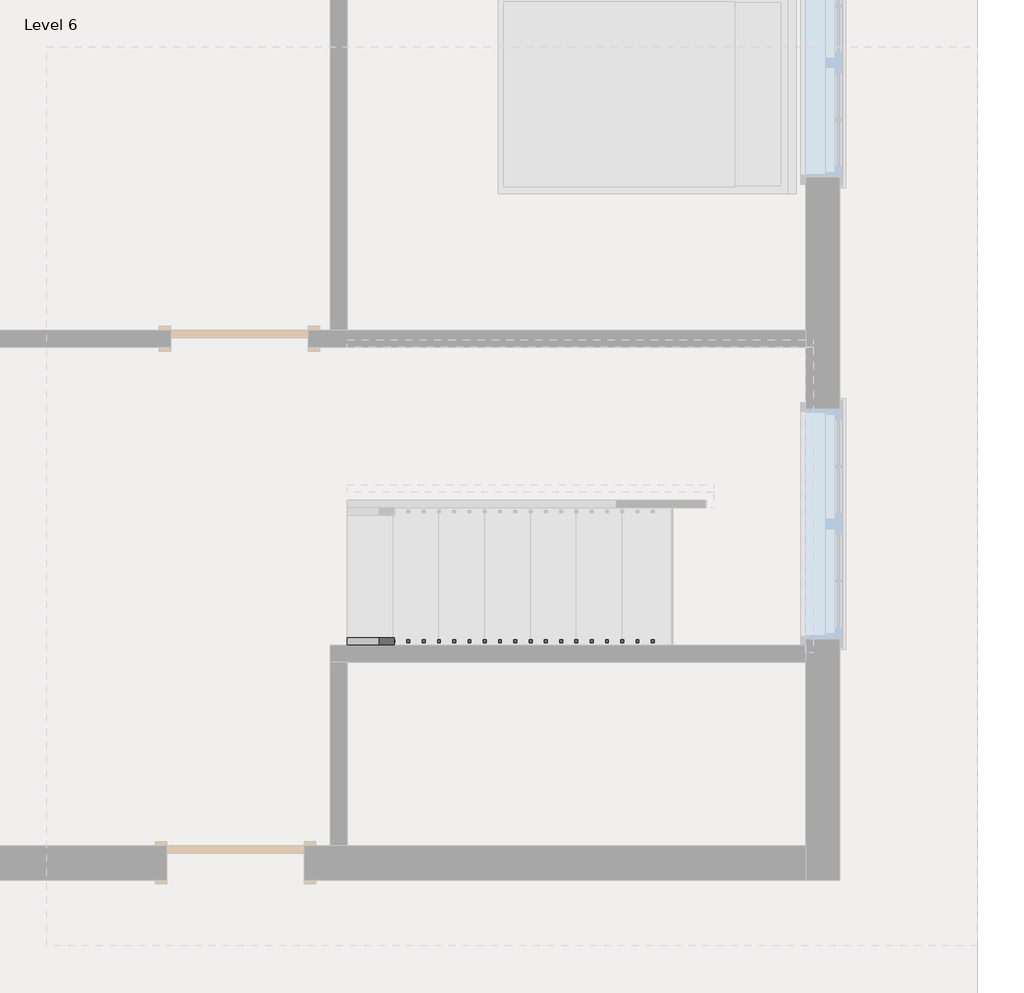
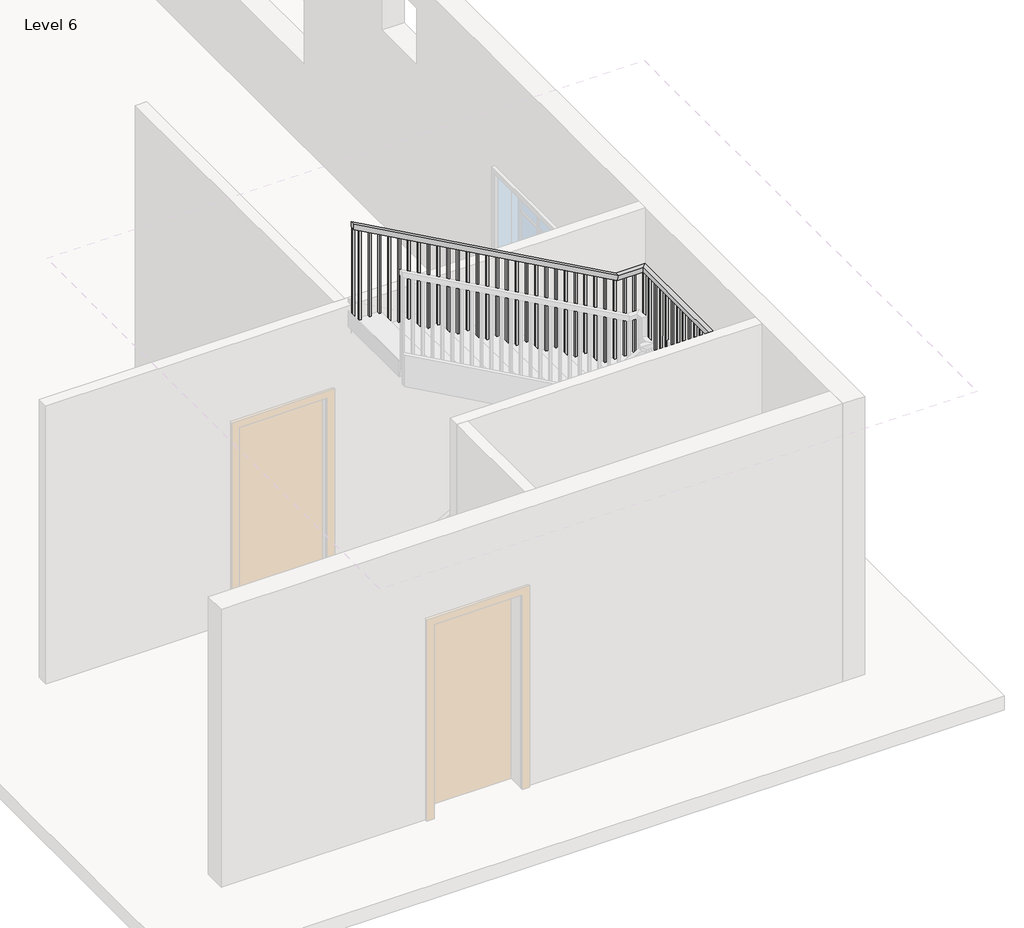
# One storey, part 2 of 3: 1 railing.
"""IFC4 building model written with IfcOpenShell, lengths in millimetres."""

from ifc_helpers import new_model, si_unit, frame, origin, place, context, project, spatial, polyline, outline, extrude, faceted_brep, element, save

model = new_model("IFC4")

# Units and contexts
model_context = context("Model", 3, world=origin())
ifc_project = project(units=[si_unit("LENGTHUNIT", "METRE", prefix="MILLI")], contexts=[model_context])

# Site, building, storey
site = spatial("IfcSite", under=ifc_project)
building = spatial("IfcBuilding", under=site)
storey = spatial("IfcBuildingStorey", under=building, Name="Level 6", Elevation=15849.6)

# Railing
placement = place(None, origin())
element("IfcRailing", 1, ObjectType="Handrail - Rectangular", at=placement, inside=storey, context=model_context, shape_type="SolidModel", body=[
    faceted_brep([(-1197.97188, -4765.70869, 16933.3333333), (-1197.97188, -4765.70869, 16875.220221), (-1197.97188, -4816.50869, 16875.220221), (-1197.97188, -4816.50869, 16933.3333333), (1240.42812, -4765.70869, 18288.0), (1253.5917222, -4765.70869, 18237.2), (1253.5917222, -4816.50869, 18237.2), (1240.42812, -4816.50869, 18288.0), (1799.22812, -4765.70869, 18288.0), (1799.22812, -4765.70869, 18237.2), (1850.02812, -4816.50869, 18237.2), (1850.02812, -4816.50869, 18288.0), (1799.22812, -2886.10869, 18288.0), (1799.22812, -2886.10869, 18237.2), (1850.02812, -2835.30869, 18237.2), (1850.02812, -2835.30869, 18288.0), (1545.22812, -2886.10869, 18288.0), (1532.0645177, -2886.10869, 18237.2), (1532.0645177, -2835.30869, 18237.2), (1545.22812, -2835.30869, 18288.0), (-1197.97188, -2886.10869, 19812.0), (-1197.97188, -2835.30869, 19812.0), (-1197.97188, -2835.30869, 19753.8868876), (-1197.97188, -2886.10869, 19753.8868876)], [[[0, 1, 2, 3]], [[1, 0, 4, 5]], [[2, 1, 5, 6]], [[3, 2, 6, 7]], [[0, 3, 7, 4]], [[5, 4, 8, 9]], [[6, 5, 9, 10]], [[7, 6, 10, 11]], [[4, 7, 11, 8]], [[9, 8, 12, 13]], [[10, 9, 13, 14]], [[11, 10, 14, 15]], [[8, 11, 15, 12]], [[13, 12, 16, 17]], [[14, 13, 17, 18]], [[15, 14, 18, 19]], [[12, 15, 19, 16]], [[20, 21, 22, 23]], [[17, 16, 20, 23]], [[18, 17, 23, 22]], [[19, 18, 22, 21]], [[16, 19, 21, 20]]]),
    extrude(outline(polyline([(19706.2618876, -1112.24688), (19716.845221, -1131.29688), (18728.2666667, -1131.29688), (18728.2666667, -1112.24688), (19706.2618876, -1112.24688)])), frame((0.0, -2870.23369, 0.0), z_axis=(0.0, 1.0, 0.0), x_axis=(0.0, 0.0, 1.0)), (0.0, 0.0, 1.0), 19.05),
    extrude(outline(polyline([(19649.8174432, -1010.64688), (19660.4007765, -1029.69688), (18728.2666667, -1029.69688), (18728.2666667, -1010.64688), (19649.8174432, -1010.64688)])), frame((0.0, -2870.23369, 0.0), z_axis=(0.0, 1.0, 0.0), x_axis=(0.0, 0.0, 1.0)), (0.0, 0.0, 1.0), 19.05),
    extrude(outline(polyline([(19593.3729988, -909.04688), (19603.9563321, -928.09688), (18728.2666667, -928.09688), (18728.2666667, -909.04688), (19593.3729988, -909.04688)])), frame((0.0, -2870.23369, 0.0), z_axis=(0.0, 1.0, 0.0), x_axis=(0.0, 0.0, 1.0)), (0.0, 0.0, 1.0), 19.05),
    extrude(outline(polyline([(19536.9285543, -807.44688), (19547.5118876, -826.49688), (18558.9333333, -826.49688), (18558.9333333, -807.44688), (19536.9285543, -807.44688)])), frame((0.0, -2870.23369, 0.0), z_axis=(0.0, 1.0, 0.0), x_axis=(0.0, 0.0, 1.0)), (0.0, 0.0, 1.0), 19.05),
    extrude(outline(polyline([(19480.4841099, -705.84688), (19491.0674432, -724.89688), (18558.9333333, -724.89688), (18558.9333333, -705.84688), (19480.4841099, -705.84688)])), frame((0.0, -2870.23369, 0.0), z_axis=(0.0, 1.0, 0.0), x_axis=(0.0, 0.0, 1.0)), (0.0, 0.0, 1.0), 19.05),
    extrude(outline(polyline([(19424.0396654, -604.24688), (19434.6229988, -623.29688), (18558.9333333, -623.29688), (18558.9333333, -604.24688), (19424.0396654, -604.24688)])), frame((0.0, -2870.23369, 0.0), z_axis=(0.0, 1.0, 0.0), x_axis=(0.0, 0.0, 1.0)), (0.0, 0.0, 1.0), 19.05),
    extrude(outline(polyline([(19367.595221, -502.64688), (19378.1785543, -521.69688), (18389.6, -521.69688), (18389.6, -502.64688), (19367.595221, -502.64688)])), frame((0.0, -2870.23369, 0.0), z_axis=(0.0, 1.0, 0.0), x_axis=(0.0, 0.0, 1.0)), (0.0, 0.0, 1.0), 19.05),
    extrude(outline(polyline([(19311.1507765, -401.04688), (19321.7341099, -420.09688), (18389.6, -420.09688), (18389.6, -401.04688), (19311.1507765, -401.04688)])), frame((0.0, -2870.23369, 0.0), z_axis=(0.0, 1.0, 0.0), x_axis=(0.0, 0.0, 1.0)), (0.0, 0.0, 1.0), 19.05),
    extrude(outline(polyline([(19254.7063321, -299.44688), (19265.2896654, -318.49688), (18389.6, -318.49688), (18389.6, -299.44688), (19254.7063321, -299.44688)])), frame((0.0, -2870.23369, 0.0), z_axis=(0.0, 1.0, 0.0), x_axis=(0.0, 0.0, 1.0)), (0.0, 0.0, 1.0), 19.05),
    extrude(outline(polyline([(19198.2618876, -197.84688), (19208.845221, -216.89688), (18220.2666667, -216.89688), (18220.2666667, -197.84688), (19198.2618876, -197.84688)])), frame((0.0, -2870.23369, 0.0), z_axis=(0.0, 1.0, 0.0), x_axis=(0.0, 0.0, 1.0)), (0.0, 0.0, 1.0), 19.05),
    extrude(outline(polyline([(19141.8174432, -96.24688), (19152.4007765, -115.29688), (18220.2666667, -115.29688), (18220.2666667, -96.24688), (19141.8174432, -96.24688)])), frame((0.0, -2870.23369, 0.0), z_axis=(0.0, 1.0, 0.0), x_axis=(0.0, 0.0, 1.0)), (0.0, 0.0, 1.0), 19.05),
    extrude(outline(polyline([(19085.3729988, 5.35312), (19095.9563321, -13.69688), (18220.2666667, -13.69688), (18220.2666667, 5.35312), (19085.3729988, 5.35312)])), frame((0.0, -2870.23369, 0.0), z_axis=(0.0, 1.0, 0.0), x_axis=(0.0, 0.0, 1.0)), (0.0, 0.0, 1.0), 19.05),
    extrude(outline(polyline([(19028.9285543, 106.95312), (19039.5118876, 87.90312), (18050.9333333, 87.90312), (18050.9333333, 106.95312), (19028.9285543, 106.95312)])), frame((0.0, -2870.23369, 0.0), z_axis=(0.0, 1.0, 0.0), x_axis=(0.0, 0.0, 1.0)), (0.0, 0.0, 1.0), 19.05),
    extrude(outline(polyline([(18972.4841099, 208.55312), (18983.0674432, 189.50312), (18050.9333333, 189.50312), (18050.9333333, 208.55312), (18972.4841099, 208.55312)])), frame((0.0, -2870.23369, 0.0), z_axis=(0.0, 1.0, 0.0), x_axis=(0.0, 0.0, 1.0)), (0.0, 0.0, 1.0), 19.05),
    extrude(outline(polyline([(18916.0396654, 310.15312), (18926.6229988, 291.10312), (18050.9333333, 291.10312), (18050.9333333, 310.15312), (18916.0396654, 310.15312)])), frame((0.0, -2870.23369, 0.0), z_axis=(0.0, 1.0, 0.0), x_axis=(0.0, 0.0, 1.0)), (0.0, 0.0, 1.0), 19.05),
    extrude(outline(polyline([(18859.595221, 411.75312), (18870.1785543, 392.70312), (17881.6, 392.70312), (17881.6, 411.75312), (18859.595221, 411.75312)])), frame((0.0, -2870.23369, 0.0), z_axis=(0.0, 1.0, 0.0), x_axis=(0.0, 0.0, 1.0)), (0.0, 0.0, 1.0), 19.05),
    extrude(outline(polyline([(18803.1507765, 513.35312), (18813.7341099, 494.30312), (17881.6, 494.30312), (17881.6, 513.35312), (18803.1507765, 513.35312)])), frame((0.0, -2870.23369, 0.0), z_axis=(0.0, 1.0, 0.0), x_axis=(0.0, 0.0, 1.0)), (0.0, 0.0, 1.0), 19.05),
    extrude(outline(polyline([(18746.7063321, 614.95312), (18757.2896654, 595.90312), (17881.6, 595.90312), (17881.6, 614.95312), (18746.7063321, 614.95312)])), frame((0.0, -2870.23369, 0.0), z_axis=(0.0, 1.0, 0.0), x_axis=(0.0, 0.0, 1.0)), (0.0, 0.0, 1.0), 19.05),
    extrude(outline(polyline([(18690.2618876, 716.55312), (18700.845221, 697.50312), (17712.2666667, 697.50312), (17712.2666667, 716.55312), (18690.2618876, 716.55312)])), frame((0.0, -2870.23369, 0.0), z_axis=(0.0, 1.0, 0.0), x_axis=(0.0, 0.0, 1.0)), (0.0, 0.0, 1.0), 19.05),
    extrude(outline(polyline([(18633.8174432, 818.15312), (18644.4007765, 799.10312), (17712.2666667, 799.10312), (17712.2666667, 818.15312), (18633.8174432, 818.15312)])), frame((0.0, -2870.23369, 0.0), z_axis=(0.0, 1.0, 0.0), x_axis=(0.0, 0.0, 1.0)), (0.0, 0.0, 1.0), 19.05),
    extrude(outline(polyline([(18577.3729988, 919.75312), (18587.9563321, 900.70312), (17712.2666667, 900.70312), (17712.2666667, 919.75312), (18577.3729988, 919.75312)])), frame((0.0, -2870.23369, 0.0), z_axis=(0.0, 1.0, 0.0), x_axis=(0.0, 0.0, 1.0)), (0.0, 0.0, 1.0), 19.05),
    extrude(outline(polyline([(18520.9285543, 1021.35312), (18531.5118876, 1002.30312), (17542.9333333, 1002.30312), (17542.9333333, 1021.35312), (18520.9285543, 1021.35312)])), frame((0.0, -2870.23369, 0.0), z_axis=(0.0, 1.0, 0.0), x_axis=(0.0, 0.0, 1.0)), (0.0, 0.0, 1.0), 19.05),
    extrude(outline(polyline([(18464.4841099, 1122.95312), (18475.0674432, 1103.90312), (17542.9333333, 1103.90312), (17542.9333333, 1122.95312), (18464.4841099, 1122.95312)])), frame((0.0, -2870.23369, 0.0), z_axis=(0.0, 1.0, 0.0), x_axis=(0.0, 0.0, 1.0)), (0.0, 0.0, 1.0), 19.05),
    extrude(outline(polyline([(18408.0396654, 1224.55312), (18418.6229988, 1205.50312), (17542.9333333, 1205.50312), (17542.9333333, 1224.55312), (18408.0396654, 1224.55312)])), frame((0.0, -2870.23369, 0.0), z_axis=(0.0, 1.0, 0.0), x_axis=(0.0, 0.0, 1.0)), (0.0, 0.0, 1.0), 19.05),
    extrude(outline(polyline([(18351.595221, 1326.15312), (18362.1785543, 1307.10312), (17373.6, 1307.10312), (17373.6, 1326.15312), (18351.595221, 1326.15312)])), frame((0.0, -2870.23369, 0.0), z_axis=(0.0, 1.0, 0.0), x_axis=(0.0, 0.0, 1.0)), (0.0, 0.0, 1.0), 19.05),
    extrude(outline(polyline([(18295.1507765, 1427.75312), (18305.7341099, 1408.70312), (17373.6, 1408.70312), (17373.6, 1427.75312), (18295.1507765, 1427.75312)])), frame((0.0, -2870.23369, 0.0), z_axis=(0.0, 1.0, 0.0), x_axis=(0.0, 0.0, 1.0)), (0.0, 0.0, 1.0), 19.05),
    extrude(outline(polyline([(18238.7063321, 1529.35312), (18249.2896654, 1510.30312), (17373.6, 1510.30312), (17373.6, 1529.35312), (18238.7063321, 1529.35312)])), frame((0.0, -2870.23369, 0.0), z_axis=(0.0, 1.0, 0.0), x_axis=(0.0, 0.0, 1.0)), (0.0, 0.0, 1.0), 19.05),
    extrude(outline(polyline([(1630.95312, -2851.18369), (1630.95312, -2870.23369), (1611.90312, -2870.23369), (1611.90312, -2851.18369), (1630.95312, -2851.18369)])), frame((0.0, 0.0, 17373.6), z_axis=(0.0, 0.0, 1.0), x_axis=(1.0, 0.0, 0.0)), (0.0, 0.0, 1.0), 863.6),
    extrude(outline(polyline([(1732.55312, -2851.18369), (1732.55312, -2870.23369), (1713.50312, -2870.23369), (1713.50312, -2851.18369), (1732.55312, -2851.18369)])), frame((0.0, 0.0, 17373.6), z_axis=(0.0, 0.0, 1.0), x_axis=(1.0, 0.0, 0.0)), (0.0, 0.0, 1.0), 863.6),
    extrude(outline(polyline([(1834.15312, -2971.83369), (1815.10312, -2971.83369), (1815.10312, -2952.78369), (1834.15312, -2952.78369), (1834.15312, -2971.83369)])), frame((0.0, 0.0, 17373.6), z_axis=(0.0, 0.0, 1.0), x_axis=(1.0, 0.0, 0.0)), (0.0, 0.0, 1.0), 863.6),
    extrude(outline(polyline([(1834.15312, -3073.43369), (1815.10312, -3073.43369), (1815.10312, -3054.38369), (1834.15312, -3054.38369), (1834.15312, -3073.43369)])), frame((0.0, 0.0, 17373.6), z_axis=(0.0, 0.0, 1.0), x_axis=(1.0, 0.0, 0.0)), (0.0, 0.0, 1.0), 863.6),
    extrude(outline(polyline([(1834.15312, -3175.03369), (1815.10312, -3175.03369), (1815.10312, -3155.98369), (1834.15312, -3155.98369), (1834.15312, -3175.03369)])), frame((0.0, 0.0, 17373.6), z_axis=(0.0, 0.0, 1.0), x_axis=(1.0, 0.0, 0.0)), (0.0, 0.0, 1.0), 863.6),
    extrude(outline(polyline([(1834.15312, -3276.63369), (1815.10312, -3276.63369), (1815.10312, -3257.58369), (1834.15312, -3257.58369), (1834.15312, -3276.63369)])), frame((0.0, 0.0, 17373.6), z_axis=(0.0, 0.0, 1.0), x_axis=(1.0, 0.0, 0.0)), (0.0, 0.0, 1.0), 863.6),
    extrude(outline(polyline([(1834.15312, -3378.23369), (1815.10312, -3378.23369), (1815.10312, -3359.18369), (1834.15312, -3359.18369), (1834.15312, -3378.23369)])), frame((0.0, 0.0, 17373.6), z_axis=(0.0, 0.0, 1.0), x_axis=(1.0, 0.0, 0.0)), (0.0, 0.0, 1.0), 863.6),
    extrude(outline(polyline([(1834.15312, -3479.83369), (1815.10312, -3479.83369), (1815.10312, -3460.78369), (1834.15312, -3460.78369), (1834.15312, -3479.83369)])), frame((0.0, 0.0, 17373.6), z_axis=(0.0, 0.0, 1.0), x_axis=(1.0, 0.0, 0.0)), (0.0, 0.0, 1.0), 863.6),
    extrude(outline(polyline([(1834.15312, -3581.43369), (1815.10312, -3581.43369), (1815.10312, -3562.38369), (1834.15312, -3562.38369), (1834.15312, -3581.43369)])), frame((0.0, 0.0, 17373.6), z_axis=(0.0, 0.0, 1.0), x_axis=(1.0, 0.0, 0.0)), (0.0, 0.0, 1.0), 863.6),
    extrude(outline(polyline([(1834.15312, -3683.03369), (1815.10312, -3683.03369), (1815.10312, -3663.98369), (1834.15312, -3663.98369), (1834.15312, -3683.03369)])), frame((0.0, 0.0, 17373.6), z_axis=(0.0, 0.0, 1.0), x_axis=(1.0, 0.0, 0.0)), (0.0, 0.0, 1.0), 863.6),
    extrude(outline(polyline([(1834.15312, -3784.63369), (1815.10312, -3784.63369), (1815.10312, -3765.58369), (1834.15312, -3765.58369), (1834.15312, -3784.63369)])), frame((0.0, 0.0, 17373.6), z_axis=(0.0, 0.0, 1.0), x_axis=(1.0, 0.0, 0.0)), (0.0, 0.0, 1.0), 863.6),
    extrude(outline(polyline([(1834.15312, -3886.23369), (1815.10312, -3886.23369), (1815.10312, -3867.18369), (1834.15312, -3867.18369), (1834.15312, -3886.23369)])), frame((0.0, 0.0, 17373.6), z_axis=(0.0, 0.0, 1.0), x_axis=(1.0, 0.0, 0.0)), (0.0, 0.0, 1.0), 863.6),
    extrude(outline(polyline([(1834.15312, -3987.83369), (1815.10312, -3987.83369), (1815.10312, -3968.78369), (1834.15312, -3968.78369), (1834.15312, -3987.83369)])), frame((0.0, 0.0, 17373.6), z_axis=(0.0, 0.0, 1.0), x_axis=(1.0, 0.0, 0.0)), (0.0, 0.0, 1.0), 863.6),
    extrude(outline(polyline([(1834.15312, -4089.43369), (1815.10312, -4089.43369), (1815.10312, -4070.38369), (1834.15312, -4070.38369), (1834.15312, -4089.43369)])), frame((0.0, 0.0, 17373.6), z_axis=(0.0, 0.0, 1.0), x_axis=(1.0, 0.0, 0.0)), (0.0, 0.0, 1.0), 863.6),
    extrude(outline(polyline([(1834.15312, -4191.03369), (1815.10312, -4191.03369), (1815.10312, -4171.98369), (1834.15312, -4171.98369), (1834.15312, -4191.03369)])), frame((0.0, 0.0, 17373.6), z_axis=(0.0, 0.0, 1.0), x_axis=(1.0, 0.0, 0.0)), (0.0, 0.0, 1.0), 863.6),
    extrude(outline(polyline([(1834.15312, -4292.63369), (1815.10312, -4292.63369), (1815.10312, -4273.58369), (1834.15312, -4273.58369), (1834.15312, -4292.63369)])), frame((0.0, 0.0, 17373.6), z_axis=(0.0, 0.0, 1.0), x_axis=(1.0, 0.0, 0.0)), (0.0, 0.0, 1.0), 863.6),
    extrude(outline(polyline([(1834.15312, -4394.23369), (1815.10312, -4394.23369), (1815.10312, -4375.18369), (1834.15312, -4375.18369), (1834.15312, -4394.23369)])), frame((0.0, 0.0, 17373.6), z_axis=(0.0, 0.0, 1.0), x_axis=(1.0, 0.0, 0.0)), (0.0, 0.0, 1.0), 863.6),
    extrude(outline(polyline([(1834.15312, -4495.83369), (1815.10312, -4495.83369), (1815.10312, -4476.78369), (1834.15312, -4476.78369), (1834.15312, -4495.83369)])), frame((0.0, 0.0, 17373.6), z_axis=(0.0, 0.0, 1.0), x_axis=(1.0, 0.0, 0.0)), (0.0, 0.0, 1.0), 863.6),
    extrude(outline(polyline([(1834.15312, -4597.43369), (1815.10312, -4597.43369), (1815.10312, -4578.38369), (1834.15312, -4578.38369), (1834.15312, -4597.43369)])), frame((0.0, 0.0, 17373.6), z_axis=(0.0, 0.0, 1.0), x_axis=(1.0, 0.0, 0.0)), (0.0, 0.0, 1.0), 863.6),
    extrude(outline(polyline([(1834.15312, -4699.03369), (1815.10312, -4699.03369), (1815.10312, -4679.98369), (1834.15312, -4679.98369), (1834.15312, -4699.03369)])), frame((0.0, 0.0, 17373.6), z_axis=(0.0, 0.0, 1.0), x_axis=(1.0, 0.0, 0.0)), (0.0, 0.0, 1.0), 863.6),
    extrude(outline(polyline([(1738.90312, -4800.63369), (1738.90312, -4781.58369), (1757.95312, -4781.58369), (1757.95312, -4800.63369), (1738.90312, -4800.63369)])), frame((0.0, 0.0, 17373.6), z_axis=(0.0, 0.0, 1.0), x_axis=(1.0, 0.0, 0.0)), (0.0, 0.0, 1.0), 863.6),
    extrude(outline(polyline([(1637.30312, -4800.63369), (1637.30312, -4781.58369), (1656.35312, -4781.58369), (1656.35312, -4800.63369), (1637.30312, -4800.63369)])), frame((0.0, 0.0, 17373.6), z_axis=(0.0, 0.0, 1.0), x_axis=(1.0, 0.0, 0.0)), (0.0, 0.0, 1.0), 863.6),
    extrude(outline(polyline([(1535.70312, -4800.63369), (1535.70312, -4781.58369), (1554.75312, -4781.58369), (1554.75312, -4800.63369), (1535.70312, -4800.63369)])), frame((0.0, 0.0, 17373.6), z_axis=(0.0, 0.0, 1.0), x_axis=(1.0, 0.0, 0.0)), (0.0, 0.0, 1.0), 863.6),
    extrude(outline(polyline([(1434.10312, -4800.63369), (1434.10312, -4781.58369), (1453.15312, -4781.58369), (1453.15312, -4800.63369), (1434.10312, -4800.63369)])), frame((0.0, 0.0, 17373.6), z_axis=(0.0, 0.0, 1.0), x_axis=(1.0, 0.0, 0.0)), (0.0, 0.0, 1.0), 863.6),
    extrude(outline(polyline([(1332.50312, -4800.63369), (1332.50312, -4781.58369), (1351.55312, -4781.58369), (1351.55312, -4800.63369), (1332.50312, -4800.63369)])), frame((0.0, 0.0, 17373.6), z_axis=(0.0, 0.0, 1.0), x_axis=(1.0, 0.0, 0.0)), (0.0, 0.0, 1.0), 863.6),
    extrude(outline(polyline([(18235.1785543, 1249.95312), (18224.595221, 1230.90312), (17373.6, 1230.90312), (17373.6, 1249.95312), (18235.1785543, 1249.95312)])), frame((0.0, -4800.63369, 0.0), z_axis=(0.0, 1.0, 0.0), x_axis=(0.0, 0.0, 1.0)), (0.0, 0.0, 1.0), 19.05),
    extrude(outline(polyline([(18178.7341099, 1148.35312), (18168.1507765, 1129.30312), (17204.2666667, 1129.30312), (17204.2666667, 1148.35312), (18178.7341099, 1148.35312)])), frame((0.0, -4800.63369, 0.0), z_axis=(0.0, 1.0, 0.0), x_axis=(0.0, 0.0, 1.0)), (0.0, 0.0, 1.0), 19.05),
    extrude(outline(polyline([(18122.2896654, 1046.75312), (18111.7063321, 1027.70312), (17204.2666667, 1027.70312), (17204.2666667, 1046.75312), (18122.2896654, 1046.75312)])), frame((0.0, -4800.63369, 0.0), z_axis=(0.0, 1.0, 0.0), x_axis=(0.0, 0.0, 1.0)), (0.0, 0.0, 1.0), 19.05),
    extrude(outline(polyline([(18065.845221, 945.15312), (18055.2618876, 926.10312), (17204.2666667, 926.10312), (17204.2666667, 945.15312), (18065.845221, 945.15312)])), frame((0.0, -4800.63369, 0.0), z_axis=(0.0, 1.0, 0.0), x_axis=(0.0, 0.0, 1.0)), (0.0, 0.0, 1.0), 19.05),
    extrude(outline(polyline([(18009.4007765, 843.55312), (17998.8174432, 824.50312), (17034.9333333, 824.50312), (17034.9333333, 843.55312), (18009.4007765, 843.55312)])), frame((0.0, -4800.63369, 0.0), z_axis=(0.0, 1.0, 0.0), x_axis=(0.0, 0.0, 1.0)), (0.0, 0.0, 1.0), 19.05),
    extrude(outline(polyline([(17952.9563321, 741.95312), (17942.3729988, 722.90312), (17034.9333333, 722.90312), (17034.9333333, 741.95312), (17952.9563321, 741.95312)])), frame((0.0, -4800.63369, 0.0), z_axis=(0.0, 1.0, 0.0), x_axis=(0.0, 0.0, 1.0)), (0.0, 0.0, 1.0), 19.05),
    extrude(outline(polyline([(17896.5118876, 640.35312), (17885.9285543, 621.30312), (17034.9333333, 621.30312), (17034.9333333, 640.35312), (17896.5118876, 640.35312)])), frame((0.0, -4800.63369, 0.0), z_axis=(0.0, 1.0, 0.0), x_axis=(0.0, 0.0, 1.0)), (0.0, 0.0, 1.0), 19.05),
    extrude(outline(polyline([(17840.0674432, 538.75312), (17829.4841099, 519.70312), (16865.6, 519.70312), (16865.6, 538.75312), (17840.0674432, 538.75312)])), frame((0.0, -4800.63369, 0.0), z_axis=(0.0, 1.0, 0.0), x_axis=(0.0, 0.0, 1.0)), (0.0, 0.0, 1.0), 19.05),
    extrude(outline(polyline([(17783.6229988, 437.15312), (17773.0396654, 418.10312), (16865.6, 418.10312), (16865.6, 437.15312), (17783.6229988, 437.15312)])), frame((0.0, -4800.63369, 0.0), z_axis=(0.0, 1.0, 0.0), x_axis=(0.0, 0.0, 1.0)), (0.0, 0.0, 1.0), 19.05),
    extrude(outline(polyline([(17727.1785543, 335.55312), (17716.595221, 316.50312), (16865.6, 316.50312), (16865.6, 335.55312), (17727.1785543, 335.55312)])), frame((0.0, -4800.63369, 0.0), z_axis=(0.0, 1.0, 0.0), x_axis=(0.0, 0.0, 1.0)), (0.0, 0.0, 1.0), 19.05),
    extrude(outline(polyline([(17670.7341099, 233.95312), (17660.1507765, 214.90312), (16696.2666667, 214.90312), (16696.2666667, 233.95312), (17670.7341099, 233.95312)])), frame((0.0, -4800.63369, 0.0), z_axis=(0.0, 1.0, 0.0), x_axis=(0.0, 0.0, 1.0)), (0.0, 0.0, 1.0), 19.05),
    extrude(outline(polyline([(17614.2896654, 132.35312), (17603.7063321, 113.30312), (16696.2666667, 113.30312), (16696.2666667, 132.35312), (17614.2896654, 132.35312)])), frame((0.0, -4800.63369, 0.0), z_axis=(0.0, 1.0, 0.0), x_axis=(0.0, 0.0, 1.0)), (0.0, 0.0, 1.0), 19.05),
    extrude(outline(polyline([(17557.845221, 30.75312), (17547.2618876, 11.70312), (16696.2666667, 11.70312), (16696.2666667, 30.75312), (17557.845221, 30.75312)])), frame((0.0, -4800.63369, 0.0), z_axis=(0.0, 1.0, 0.0), x_axis=(0.0, 0.0, 1.0)), (0.0, 0.0, 1.0), 19.05),
    extrude(outline(polyline([(17501.4007765, -70.84688), (17490.8174432, -89.89688), (16526.9333333, -89.89688), (16526.9333333, -70.84688), (17501.4007765, -70.84688)])), frame((0.0, -4800.63369, 0.0), z_axis=(0.0, 1.0, 0.0), x_axis=(0.0, 0.0, 1.0)), (0.0, 0.0, 1.0), 19.05),
    extrude(outline(polyline([(17444.9563321, -172.44688), (17434.3729988, -191.49688), (16526.9333333, -191.49688), (16526.9333333, -172.44688), (17444.9563321, -172.44688)])), frame((0.0, -4800.63369, 0.0), z_axis=(0.0, 1.0, 0.0), x_axis=(0.0, 0.0, 1.0)), (0.0, 0.0, 1.0), 19.05),
    extrude(outline(polyline([(17388.5118876, -274.04688), (17377.9285543, -293.09688), (16526.9333333, -293.09688), (16526.9333333, -274.04688), (17388.5118876, -274.04688)])), frame((0.0, -4800.63369, 0.0), z_axis=(0.0, 1.0, 0.0), x_axis=(0.0, 0.0, 1.0)), (0.0, 0.0, 1.0), 19.05),
    extrude(outline(polyline([(17332.0674432, -375.64688), (17321.4841099, -394.69688), (16357.6, -394.69688), (16357.6, -375.64688), (17332.0674432, -375.64688)])), frame((0.0, -4800.63369, 0.0), z_axis=(0.0, 1.0, 0.0), x_axis=(0.0, 0.0, 1.0)), (0.0, 0.0, 1.0), 19.05),
    extrude(outline(polyline([(17275.6229988, -477.24688), (17265.0396654, -496.29688), (16357.6, -496.29688), (16357.6, -477.24688), (17275.6229988, -477.24688)])), frame((0.0, -4800.63369, 0.0), z_axis=(0.0, 1.0, 0.0), x_axis=(0.0, 0.0, 1.0)), (0.0, 0.0, 1.0), 19.05),
    extrude(outline(polyline([(17219.1785543, -578.84688), (17208.595221, -597.89688), (16357.6, -597.89688), (16357.6, -578.84688), (17219.1785543, -578.84688)])), frame((0.0, -4800.63369, 0.0), z_axis=(0.0, 1.0, 0.0), x_axis=(0.0, 0.0, 1.0)), (0.0, 0.0, 1.0), 19.05),
    extrude(outline(polyline([(17162.7341099, -680.44688), (17152.1507765, -699.49688), (16188.2666667, -699.49688), (16188.2666667, -680.44688), (17162.7341099, -680.44688)])), frame((0.0, -4800.63369, 0.0), z_axis=(0.0, 1.0, 0.0), x_axis=(0.0, 0.0, 1.0)), (0.0, 0.0, 1.0), 19.05),
    extrude(outline(polyline([(17106.2896654, -782.04688), (17095.7063321, -801.09688), (16188.2666667, -801.09688), (16188.2666667, -782.04688), (17106.2896654, -782.04688)])), frame((0.0, -4800.63369, 0.0), z_axis=(0.0, 1.0, 0.0), x_axis=(0.0, 0.0, 1.0)), (0.0, 0.0, 1.0), 19.05),
    extrude(outline(polyline([(17049.845221, -883.64688), (17039.2618876, -902.69688), (16188.2666667, -902.69688), (16188.2666667, -883.64688), (17049.845221, -883.64688)])), frame((0.0, -4800.63369, 0.0), z_axis=(0.0, 1.0, 0.0), x_axis=(0.0, 0.0, 1.0)), (0.0, 0.0, 1.0), 19.05),
    extrude(outline(polyline([(16993.4007765, -985.24688), (16982.8174432, -1004.29688), (16018.9333333, -1004.29688), (16018.9333333, -985.24688), (16993.4007765, -985.24688)])), frame((0.0, -4800.63369, 0.0), z_axis=(0.0, 1.0, 0.0), x_axis=(0.0, 0.0, 1.0)), (0.0, 0.0, 1.0), 19.05),
    extrude(outline(polyline([(16936.9563321, -1086.84688), (16926.3729988, -1105.89688), (16018.9333333, -1105.89688), (16018.9333333, -1086.84688), (16936.9563321, -1086.84688)])), frame((0.0, -4800.63369, 0.0), z_axis=(0.0, 1.0, 0.0), x_axis=(0.0, 0.0, 1.0)), (0.0, 0.0, 1.0), 19.05),
    extrude(outline(polyline([(1834.15312, -2870.23369), (1815.10312, -2870.23369), (1815.10312, -2851.18369), (1834.15312, -2851.18369), (1834.15312, -2870.23369)])), frame((0.0, 0.0, 17373.6), z_axis=(0.0, 0.0, 1.0), x_axis=(1.0, 0.0, 0.0)), (0.0, 0.0, 1.0), 863.6),
    extrude(outline(polyline([(1815.10312, -4800.63369), (1815.10312, -4781.58369), (1834.15312, -4781.58369), (1834.15312, -4800.63369), (1815.10312, -4800.63369)])), frame((0.0, 0.0, 17373.6), z_axis=(0.0, 0.0, 1.0), x_axis=(1.0, 0.0, 0.0)), (0.0, 0.0, 1.0), 863.6),
    extrude(outline(polyline([(19743.3035543, -1178.92188), (19753.8868876, -1197.97188), (18728.2666667, -1197.97188), (18728.2666667, -1178.92188), (19743.3035543, -1178.92188)])), frame((0.0, -2870.23369, 0.0), z_axis=(0.0, 1.0, 0.0), x_axis=(0.0, 0.0, 1.0)), (0.0, 0.0, 1.0), 19.05),
    extrude(outline(polyline([(16885.8035543, -1178.92188), (16875.220221, -1197.97188), (16018.9333333, -1197.97188), (16018.9333333, -1178.92188), (16885.8035543, -1178.92188)])), frame((0.0, -4800.63369, 0.0), z_axis=(0.0, 1.0, 0.0), x_axis=(0.0, 0.0, 1.0)), (0.0, 0.0, 1.0), 19.05),
])

save(model, "model.ifc")

# Revit data of these elements
# Type "Handrail - Rectangular"
#   Assembly Code = "C2010400"
#   built-in parameter 1008612 = 0.0416667 (stored number, unit not read)
#   built-in parameter 1008611 = 0.0416667 (stored number, unit not read)
#   built-in parameter 1008609 = 0.333333 (stored number, unit not read)
#   built-in parameter 1008604 = 0.166667 (stored number, unit not read)
#   built-in parameter 1008603 = 0.166667 (stored number, unit not read)
#   Railing Height = 3' - 0"
#   built-in parameter 1008630 = 2
#   built-in parameter 1008610 = 2
#   built-in parameter 1008618 = Baluster - Square : 3/4"
# Element 1 (IfcRailing, "Handrail - Rectangular")
#   Phase Created = New Construction
